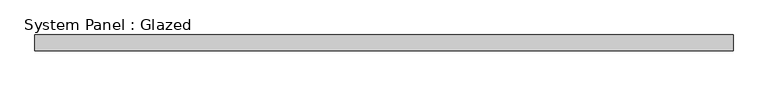
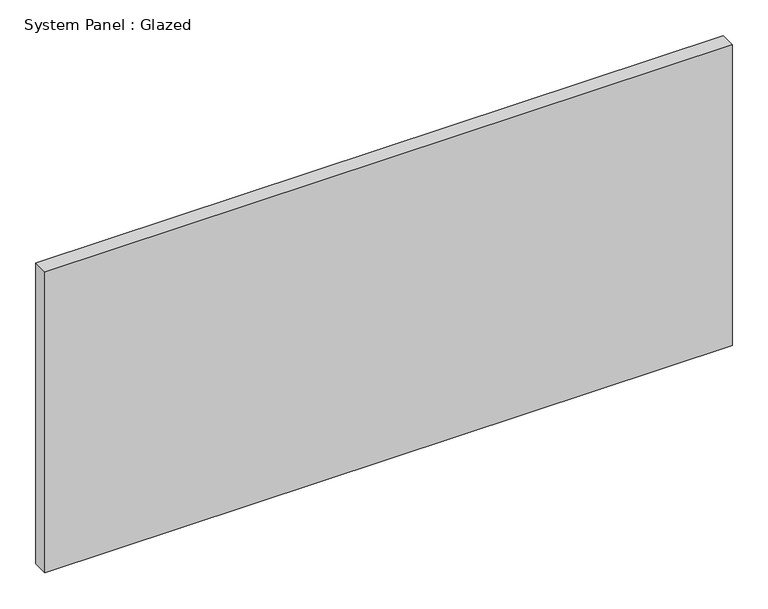
"""IFC4 building model written with IfcOpenShell, lengths in millimetres: plate geometry, System Panel : Glazed."""

from ifc_helpers import new_model, si_unit, origin, origin_with_axes, place, context, project, spatial, polyline, outline, extrude, source, transform, mapped, element, save


def system_panel_glazed_3c79bf9a(model_context):
    return source(origin(), model_context, "Body", "SweptSolid", [
        extrude(outline(polyline([(555.625, -44.45), (-555.625, -44.45), (-555.625, -19.05), (555.625, -19.05), (555.625, -44.45)])), origin_with_axes(), (0.0, 0.0, 1.0), 514.35),
    ])


if __name__ == "__main__":
    model = new_model("IFC4")
    model_context = context("Model", 3, world=origin())
    ifc_project = project(units=[si_unit("LENGTHUNIT", "METRE", prefix="MILLI")], contexts=[model_context])
    site = spatial("IfcSite", under=ifc_project)
    building = spatial("IfcBuilding", under=site)
    placement = place(None, origin())
    system_panel_glazed_shape = system_panel_glazed_3c79bf9a(model_context)
    element("IfcPlate", 1, ObjectType="System Panel : Glazed", at=placement, inside=building, context=model_context, shape_type="MappedRepresentation", body=[
        mapped(system_panel_glazed_shape, transform((0.0, 0.0, 0.0), x_axis=(1.0, 0.0, 0.0), y_axis=(0.0, 1.0, 0.0), z_axis=(0.0, 0.0, 1.0))),
    ])
    save(model, "model.ifc")

# Revit data of these elements
# Type "System Panel : Glazed"
#   Construction Type Id = "GSP4R"
#   Analytic Construction = "1/8 in Pilkington single glazing"
#   Visual Light Transmittance = 0.9
#   Solar Heat Gain Coefficient = 0.86
#   Heat Transfer Coefficient (U) = 1.18115 BTU/(h·ft²·°F)
#   Define Thermal Properties by = 1
# Element 1 (IfcPlate, "System Panel : Glazed")
#   Materials on its faces: "glass panel 223"
# Materials
#   "glass panel 223": class "Generic", colour RGB 120 120 120, transparency 0, Cost = 0
